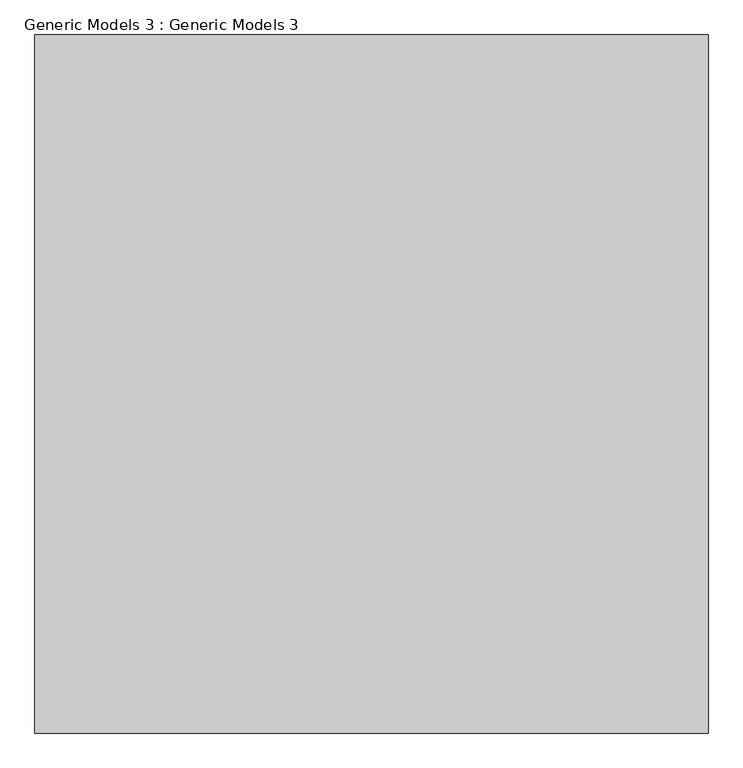
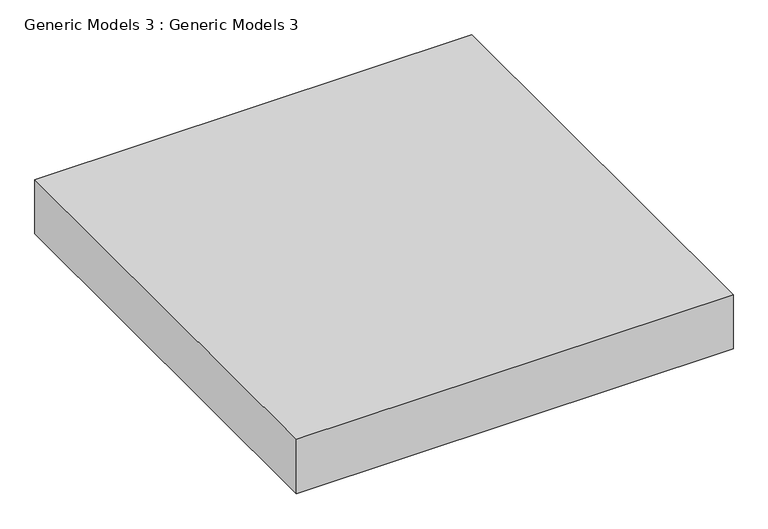
"""IFC4 building model written with IfcOpenShell, lengths in millimetres: proxy geometry, Generic Models 3 : Generic Models 3."""

from ifc_helpers import new_model, si_unit, frame, origin, place, context, project, spatial, polyline, outline, extrude, source, transform, mapped, element, save


def generic_models_3_generic_models_3_d114d96d(model_context):
    return source(origin(), model_context, "Body", "SweptSolid", [
        extrude(outline(polyline([(4979.9930105, 9998.4019701), (4979.9930105, -6007.8398788), (-10463.2069895, -6007.8398788), (-10463.2069895, 9998.4019701), (4979.9930105, 9998.4019701)])), frame((0.0, 0.0, 6400.8), z_axis=(0.0, 0.0, 1.0), x_axis=(1.0, 0.0, 0.0)), (0.0, 0.0, 1.0), 2033.9300232),
    ])


if __name__ == "__main__":
    model = new_model("IFC4")
    model_context = context("Model", 3, world=origin())
    ifc_project = project(units=[si_unit("LENGTHUNIT", "METRE", prefix="MILLI")], contexts=[model_context])
    site = spatial("IfcSite", under=ifc_project)
    building = spatial("IfcBuilding", under=site)
    placement = place(None, origin())
    generic_models_3_generic_models_3_shape = generic_models_3_generic_models_3_d114d96d(model_context)
    element("IfcBuildingElementProxy", 1, Name="Generic Models 3 : Generic Models 3", ObjectType="Generic Models 3 : Generic Models 3", at=placement, inside=building, context=model_context, shape_type="MappedRepresentation", body=[
        mapped(generic_models_3_generic_models_3_shape, transform((0.0, 0.0, 0.0), x_axis=(1.0, 0.0, 0.0), y_axis=(0.0, 1.0, 0.0), z_axis=(0.0, 0.0, 1.0))),
    ])
    save(model, "model.ifc")
